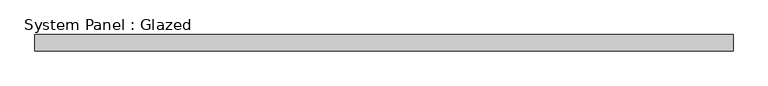
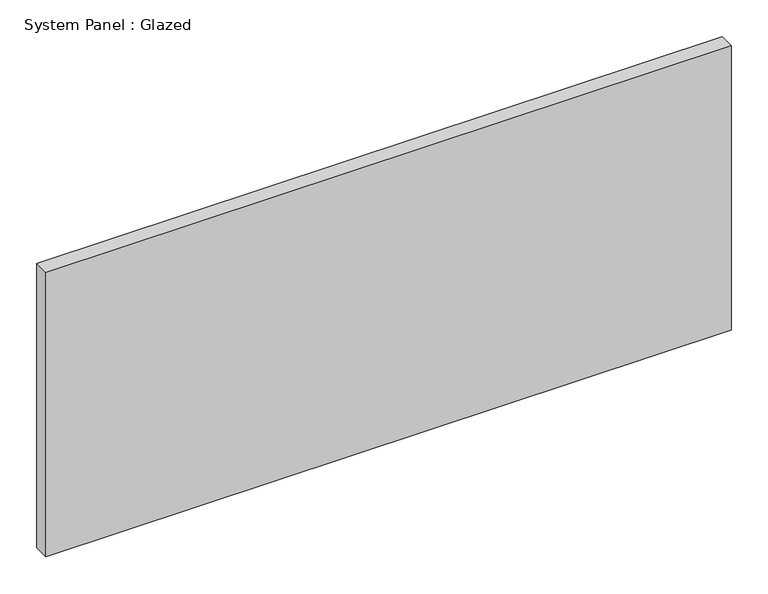
"""IFC4 building model written with IfcOpenShell, lengths in millimetres: plate geometry, System Panel : Glazed."""

from ifc_helpers import new_model, si_unit, origin, origin_with_axes, place, context, project, spatial, polyline, outline, extrude, source, transform, mapped, element, save


def system_panel_glazed_a8ba4957(model_context):
    return source(origin(), model_context, "Body", "SweptSolid", [
        extrude(outline(polyline([(539.75, 19.05), (-539.75, 19.05), (-539.75, 44.45), (539.75, 44.45), (539.75, 19.05)])), origin_with_axes(), (0.0, 0.0, 1.0), 473.71),
    ])


if __name__ == "__main__":
    model = new_model("IFC4")
    model_context = context("Model", 3, world=origin())
    ifc_project = project(units=[si_unit("LENGTHUNIT", "METRE", prefix="MILLI")], contexts=[model_context])
    site = spatial("IfcSite", under=ifc_project)
    building = spatial("IfcBuilding", under=site)
    placement = place(None, origin())
    system_panel_glazed_shape = system_panel_glazed_a8ba4957(model_context)
    element("IfcPlate", 1, ObjectType="System Panel : Glazed", at=placement, inside=building, context=model_context, shape_type="MappedRepresentation", body=[
        mapped(system_panel_glazed_shape, transform((0.0, 0.0, 0.0), x_axis=(1.0, 0.0, 0.0), y_axis=(0.0, 1.0, 0.0), z_axis=(0.0, 0.0, 1.0))),
    ])
    save(model, "model.ifc")

# Revit data of these elements
# Type "System Panel : Glazed"
#   Construction Type Id = "GSP4R"
#   Analytic Construction = "1/8 in Pilkington single glazing"
#   Visual Light Transmittance = 0.9
#   Solar Heat Gain Coefficient = 0.86
#   Heat Transfer Coefficient (U) = 1.18115 BTU/(h·ft²·°F)
#   Define Thermal Properties by = 1
# Element 1 (IfcPlate, "System Panel : Glazed")
#   Materials on its faces: "Glass"
# Materials
#   "Glass": class "Glass", colour RGB 0 128 192, transparency 0.75, Description = "Soda Lime Glass", Cost = 0
